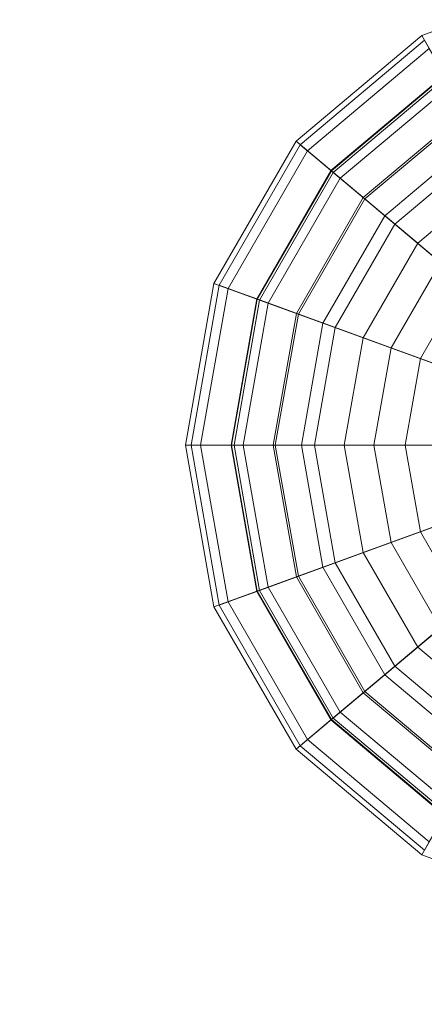
# Model space of a CAD drawing. Units: inches. Extents: x 375 to 1122, y 27 to 1069.
# Tile 97 of 155: x 717.434 to 718.593, y 863.668 to 866.486. Entities that reach past the tile are written whole.
import ezdxf

# ---------------------------------------------------------------- set-up
doc = ezdxf.new("R2010")
doc.units = ezdxf.units.IN
doc.layers.add('A-ANNO-DIMS', color=2, linetype='Continuous', lineweight=18)
doc.layers.add('Furniture', color=30, linetype='Continuous', lineweight=18)
doc.styles.get("Standard").update_dxf_attribs({"font": 'arial.ttf'})
doc.dimstyles.new('ISO-25', dxfattribs={"dimtxt": 12, "dimasz": 2.5, "dimexe": 1.5, "dimexo": 1.5, "dimtad": 1, "dimdec": 1, "dimlunit": 3, "dimtxsty": 'Standard', "dimblk": 'ARCHTICK', "dimcen": 2.5, "dimadec": 0, "dimazin": 0, "dimtfac": 1, "dimtdec": 1, "dimtmove": 0, "dimatfit": 3, "dimfxl": 1.5, "dimfxlon": 1, "dimarcsym": 0})

# ---------------------------------------------------------------- blocks, each defined once
blk = doc.blocks.new('A$C403C54AD')
for points in [[(1.793211, 0.852004, -0.031825), (1.826559, 0.857884, -0.028747), (1.826559, 0.857884, -0.028747), (1.797233, 0.840953, -0.031825)], [(1.797233, 0.840953, -0.031825), (1.826559, 0.857884, -0.028747), (1.826559, 0.857884, -0.028747), (1.804793, 0.831944, -0.031825)], [(1.804793, 0.831944, -0.031825), (1.826559, 0.857884, -0.028747), (1.826559, 0.857884, -0.028747), (1.814977, 0.826064, -0.031825)], [(1.814977, 0.826064, -0.031825), (1.826559, 0.857884, -0.028747), (1.826559, 0.857884, -0.028747), (1.826559, 0.824022, -0.031825)], [(1.855884, 0.840953, -0.031825), (1.826559, 0.857884, -0.028747), (1.826559, 0.857884, -0.028747), (1.859907, 0.852004, -0.031825)], [(1.848325, 0.831944, -0.031825), (1.826559, 0.857884, -0.028747), (1.826559, 0.857884, -0.028747), (1.855884, 0.840953, -0.031825)], [(1.83814, 0.826064, -0.031825), (1.826559, 0.857884, -0.028747), (1.826559, 0.857884, -0.028747), (1.848325, 0.831944, -0.031825)], [(1.826559, 0.824022, -0.031825), (1.826559, 0.857884, -0.028747), (1.826559, 0.857884, -0.028747), (1.83814, 0.826064, -0.031825)], [(1.796427, 0.852571, -0.028594), (1.793211, 0.852004, -0.031825), (1.797233, 0.840953, -0.031825), (1.800062, 0.842586, -0.028594)], [(1.853056, 0.842586, -0.028594), (1.855884, 0.840953, -0.031825), (1.859907, 0.852004, -0.031825), (1.85669, 0.852571, -0.028594)], [(1.814249, 0.850777, -0.02532), (1.800062, 0.842586, -0.028594), (1.806892, 0.834446, -0.028594), (1.817422, 0.846995, -0.02532)], [(1.820835, 0.851063, 0.057003), (1.814907, 0.843998, 0.063639), (1.820359, 0.84085, 0.063639), (1.823514, 0.849517, 0.057003)], [(1.829604, 0.849517, 0.057003), (1.832759, 0.84085, 0.063639), (1.838211, 0.843998, 0.063639), (1.832282, 0.851063, 0.057003)], [(1.835696, 0.846995, -0.02532), (1.846226, 0.834446, -0.028594), (1.853056, 0.842586, -0.028594), (1.838869, 0.850777, -0.02532)], [(1.813473, 0.842289, 0.061451), (1.820055, 0.850133, 0.054084), (1.823098, 0.848375, 0.054084), (1.819596, 0.838754, 0.061451)], [(1.833522, 0.838754, 0.061451), (1.83002, 0.848375, 0.054084), (1.833063, 0.850133, 0.054084), (1.839644, 0.842289, 0.061451)], [(1.823514, 0.849517, 0.057003), (1.820359, 0.84085, 0.063639), (1.826559, 0.839757, 0.063639), (1.826559, 0.84898, 0.057003)], [(1.826559, 0.84898, 0.057003), (1.826559, 0.839757, 0.063639), (1.832759, 0.84085, 0.063639), (1.829604, 0.849517, 0.057003)], [(1.81086, 0.84882, 0.063639), (1.805243, 0.845577, 0.073031), (1.810738, 0.839029, 0.073031), (1.814907, 0.843998, 0.063639)], [(1.838211, 0.843998, 0.063639), (1.84238, 0.839029, 0.073031), (1.847874, 0.845577, 0.073031), (1.842258, 0.84882, 0.063639)], [(1.819596, 0.838754, 0.061451), (1.823098, 0.848375, 0.054084), (1.826559, 0.847765, 0.054084), (1.826559, 0.837526, 0.061451)], [(1.826559, 0.837526, 0.061451), (1.826559, 0.847765, 0.054084), (1.83002, 0.848375, 0.054084), (1.833522, 0.838754, 0.061451)], [(1.802809, 0.844172, 0.071684), (1.808929, 0.847705, 0.061451), (1.813473, 0.842289, 0.061451), (1.808931, 0.836876, 0.071684)], [(1.844187, 0.836876, 0.071684), (1.839644, 0.842289, 0.061451), (1.844189, 0.847705, 0.061451), (1.850309, 0.844172, 0.071684)], [(1.802683, 0.844099, 0.130354), (1.80709, 0.846643, 0.140564), (1.812108, 0.840662, 0.140564), (1.808838, 0.836765, 0.130354)], [(1.80709, 0.846643, 0.140564), (1.804424, 0.845104, 0.140564), (1.81013, 0.838304, 0.140564), (1.812108, 0.840662, 0.140564)], [(1.817422, 0.846995, -0.02532), (1.806892, 0.834446, -0.028594), (1.816094, 0.829133, -0.028594), (1.821697, 0.844527, -0.02532)], [(1.83142, 0.844527, -0.02532), (1.837023, 0.829133, -0.028594), (1.846226, 0.834446, -0.028594), (1.835696, 0.846995, -0.02532)], [(1.84101, 0.840662, 0.140564), (1.842988, 0.838304, 0.140564), (1.848694, 0.845104, 0.140564), (1.846028, 0.846643, 0.140564)], [(1.84428, 0.836765, 0.130354), (1.84101, 0.840662, 0.140564), (1.846028, 0.846643, 0.140564), (1.850434, 0.844099, 0.130354)], [(1.804424, 0.845104, 0.140564), (1.800097, 0.842606, 0.131159), (1.806918, 0.834477, 0.131159), (1.81013, 0.838304, 0.140564)], [(1.805243, 0.845577, 0.073031), (1.80082, 0.843024, 0.090178), (1.807455, 0.835117, 0.090178), (1.810738, 0.839029, 0.073031)], [(1.84238, 0.839029, 0.073031), (1.845663, 0.835117, 0.090178), (1.852298, 0.843024, 0.090178), (1.847874, 0.845577, 0.073031)], [(1.842988, 0.838304, 0.140564), (1.8462, 0.834477, 0.131159), (1.853021, 0.842606, 0.131159), (1.848694, 0.845104, 0.140564)], [(1.821697, 0.844527, -0.02532), (1.816094, 0.829133, -0.028594), (1.826559, 0.827288, -0.028594), (1.826559, 0.84367, -0.02532)], [(1.826559, 0.84367, -0.02532), (1.826559, 0.827288, -0.028594), (1.837023, 0.829133, -0.028594), (1.83142, 0.844527, -0.02532)], [(1.798163, 0.84149, 0.089693), (1.802809, 0.844172, 0.071684), (1.808931, 0.836876, 0.071684), (1.805483, 0.832767, 0.089693)], [(1.80025, 0.842695, 0.117718), (1.802683, 0.844099, 0.130354), (1.808838, 0.836765, 0.130354), (1.807032, 0.834612, 0.117718)], [(1.814907, 0.843998, 0.063639), (1.810738, 0.839029, 0.073031), (1.818141, 0.834755, 0.073031), (1.820359, 0.84085, 0.063639)], [(1.832759, 0.84085, 0.063639), (1.834977, 0.834755, 0.073031), (1.84238, 0.839029, 0.073031), (1.838211, 0.843998, 0.063639)], [(1.847635, 0.832767, 0.089693), (1.844187, 0.836876, 0.071684), (1.850309, 0.844172, 0.071684), (1.854954, 0.84149, 0.089693)], [(1.846086, 0.834612, 0.117718), (1.84428, 0.836765, 0.130354), (1.850434, 0.844099, 0.130354), (1.852868, 0.842695, 0.117718)], [(1.80082, 0.843024, 0.090178), (1.80025, 0.842695, 0.117718), (1.807032, 0.834612, 0.117718), (1.807455, 0.835117, 0.090178)], [(1.845663, 0.835117, 0.090178), (1.846086, 0.834612, 0.117718), (1.852868, 0.842695, 0.117718), (1.852298, 0.843024, 0.090178)], [(1.800062, 0.842586, -0.028594), (1.797233, 0.840953, -0.031825), (1.804793, 0.831944, -0.031825), (1.806892, 0.834446, -0.028594)], [(1.800097, 0.842606, 0.131159), (1.797579, 0.841152, 0.117935), (1.805049, 0.83225, 0.117935), (1.806918, 0.834477, 0.131159)], [(1.808931, 0.836876, 0.071684), (1.813473, 0.842289, 0.061451), (1.819596, 0.838754, 0.061451), (1.817179, 0.832114, 0.071684)], [(1.835938, 0.832114, 0.071684), (1.833522, 0.838754, 0.061451), (1.839644, 0.842289, 0.061451), (1.844187, 0.836876, 0.071684)], [(1.8462, 0.834477, 0.131159), (1.848069, 0.83225, 0.117935), (1.855539, 0.841152, 0.117935), (1.853021, 0.842606, 0.131159)], [(1.846226, 0.834446, -0.028594), (1.848325, 0.831944, -0.031825), (1.855884, 0.840953, -0.031825), (1.853056, 0.842586, -0.028594)], [(1.797579, 0.841152, 0.117935), (1.798163, 0.84149, 0.089693), (1.805483, 0.832767, 0.089693), (1.805049, 0.83225, 0.117935)], [(1.820359, 0.84085, 0.063639), (1.818141, 0.834755, 0.073031), (1.826559, 0.833271, 0.073031), (1.826559, 0.839757, 0.063639)], [(1.826559, 0.839757, 0.063639), (1.826559, 0.833271, 0.073031), (1.834977, 0.834755, 0.073031), (1.832759, 0.84085, 0.063639)], [(1.848069, 0.83225, 0.117935), (1.847635, 0.832767, 0.089693), (1.854954, 0.84149, 0.089693), (1.855539, 0.841152, 0.117935)], [(1.808838, 0.836765, 0.130354), (1.812108, 0.840662, 0.140564), (1.81887, 0.836759, 0.140564), (1.81713, 0.831977, 0.130354)], [(1.812108, 0.840662, 0.140564), (1.81013, 0.838304, 0.140564), (1.817817, 0.833866, 0.140564), (1.81887, 0.836759, 0.140564)], [(1.834248, 0.836759, 0.140564), (1.835301, 0.833866, 0.140564), (1.842988, 0.838304, 0.140564), (1.84101, 0.840662, 0.140564)], [(1.835988, 0.831977, 0.130354), (1.834248, 0.836759, 0.140564), (1.84101, 0.840662, 0.140564), (1.84428, 0.836765, 0.130354)], [(1.810738, 0.839029, 0.073031), (1.807455, 0.835117, 0.090178), (1.816394, 0.829956, 0.090178), (1.818141, 0.834755, 0.073031)], [(1.817179, 0.832114, 0.071684), (1.819596, 0.838754, 0.061451), (1.826559, 0.837526, 0.061451), (1.826559, 0.83046, 0.071684)], [(1.826559, 0.83046, 0.071684), (1.826559, 0.837526, 0.061451), (1.833522, 0.838754, 0.061451), (1.835938, 0.832114, 0.071684)], [(1.834977, 0.834755, 0.073031), (1.836724, 0.829956, 0.090178), (1.845663, 0.835117, 0.090178), (1.84238, 0.839029, 0.073031)], [(1.81013, 0.838304, 0.140564), (1.806918, 0.834477, 0.131159), (1.816108, 0.829171, 0.131159), (1.817817, 0.833866, 0.140564)], [(1.835301, 0.833866, 0.140564), (1.83701, 0.829171, 0.131159), (1.8462, 0.834477, 0.131159), (1.842988, 0.838304, 0.140564)], [(1.805483, 0.832767, 0.089693), (1.808931, 0.836876, 0.071684), (1.817179, 0.832114, 0.071684), (1.815345, 0.827073, 0.089693)], [(1.807032, 0.834612, 0.117718), (1.808838, 0.836765, 0.130354), (1.81713, 0.831977, 0.130354), (1.816169, 0.829337, 0.117718)], [(1.81713, 0.831977, 0.130354), (1.81887, 0.836759, 0.140564), (1.826559, 0.835403, 0.140564), (1.826559, 0.830315, 0.130354)], [(1.81887, 0.836759, 0.140564), (1.817817, 0.833866, 0.140564), (1.826559, 0.832324, 0.140564), (1.826559, 0.835403, 0.140564)], [(1.826559, 0.835403, 0.140564), (1.826559, 0.832324, 0.140564), (1.835301, 0.833866, 0.140564), (1.834248, 0.836759, 0.140564)], [(1.826559, 0.830315, 0.130354), (1.826559, 0.835403, 0.140564), (1.834248, 0.836759, 0.140564), (1.835988, 0.831977, 0.130354)], [(1.837773, 0.827073, 0.089693), (1.835938, 0.832114, 0.071684), (1.844187, 0.836876, 0.071684), (1.847635, 0.832767, 0.089693)], [(1.836949, 0.829337, 0.117718), (1.835988, 0.831977, 0.130354), (1.84428, 0.836765, 0.130354), (1.846086, 0.834612, 0.117718)], [(1.806892, 0.834446, -0.028594), (1.804793, 0.831944, -0.031825), (1.814977, 0.826064, -0.031825), (1.816094, 0.829133, -0.028594)], [(1.806918, 0.834477, 0.131159), (1.805049, 0.83225, 0.117935), (1.815114, 0.826439, 0.117935), (1.816108, 0.829171, 0.131159)], [(1.807455, 0.835117, 0.090178), (1.807032, 0.834612, 0.117718), (1.816169, 0.829337, 0.117718), (1.816394, 0.829956, 0.090178)], [(1.818141, 0.834755, 0.073031), (1.816394, 0.829956, 0.090178), (1.826559, 0.828163, 0.090178), (1.826559, 0.833271, 0.073031)], [(1.826559, 0.833271, 0.073031), (1.826559, 0.828163, 0.090178), (1.836724, 0.829956, 0.090178), (1.834977, 0.834755, 0.073031)], [(1.836724, 0.829956, 0.090178), (1.836949, 0.829337, 0.117718), (1.846086, 0.834612, 0.117718), (1.845663, 0.835117, 0.090178)], [(1.83701, 0.829171, 0.131159), (1.838004, 0.826439, 0.117935), (1.848069, 0.83225, 0.117935), (1.8462, 0.834477, 0.131159)], [(1.837023, 0.829133, -0.028594), (1.83814, 0.826064, -0.031825), (1.848325, 0.831944, -0.031825), (1.846226, 0.834446, -0.028594)], [(1.817817, 0.833866, 0.140564), (1.816108, 0.829171, 0.131159), (1.826559, 0.827328, 0.131159), (1.826559, 0.832324, 0.140564)], [(1.826559, 0.832324, 0.140564), (1.826559, 0.827328, 0.131159), (1.83701, 0.829171, 0.131159), (1.835301, 0.833866, 0.140564)], [(1.805049, 0.83225, 0.117935), (1.805483, 0.832767, 0.089693), (1.815345, 0.827073, 0.089693), (1.815114, 0.826439, 0.117935)], [(1.838004, 0.826439, 0.117935), (1.837773, 0.827073, 0.089693), (1.847635, 0.832767, 0.089693), (1.848069, 0.83225, 0.117935)], [(1.815345, 0.827073, 0.089693), (1.817179, 0.832114, 0.071684), (1.826559, 0.83046, 0.071684), (1.826559, 0.825096, 0.089693)], [(1.816169, 0.829337, 0.117718), (1.81713, 0.831977, 0.130354), (1.826559, 0.830315, 0.130354), (1.826559, 0.827505, 0.117718)], [(1.826559, 0.825096, 0.089693), (1.826559, 0.83046, 0.071684), (1.835938, 0.832114, 0.071684), (1.837773, 0.827073, 0.089693)], [(1.826559, 0.827505, 0.117718), (1.826559, 0.830315, 0.130354), (1.835988, 0.831977, 0.130354), (1.836949, 0.829337, 0.117718)], [(1.816394, 0.829956, 0.090178), (1.816169, 0.829337, 0.117718), (1.826559, 0.827505, 0.117718), (1.826559, 0.828163, 0.090178)], [(1.826559, 0.828163, 0.090178), (1.826559, 0.827505, 0.117718), (1.836949, 0.829337, 0.117718), (1.836724, 0.829956, 0.090178)], [(1.816094, 0.829133, -0.028594), (1.814977, 0.826064, -0.031825), (1.826559, 0.824022, -0.031825), (1.826559, 0.827288, -0.028594)], [(1.816108, 0.829171, 0.131159), (1.815114, 0.826439, 0.117935), (1.826559, 0.824421, 0.117935), (1.826559, 0.827328, 0.131159)], [(1.826559, 0.827328, 0.131159), (1.826559, 0.824421, 0.117935), (1.838004, 0.826439, 0.117935), (1.83701, 0.829171, 0.131159)], [(1.826559, 0.827288, -0.028594), (1.826559, 0.824022, -0.031825), (1.83814, 0.826064, -0.031825), (1.837023, 0.829133, -0.028594)], [(1.815114, 0.826439, 0.117935), (1.815345, 0.827073, 0.089693), (1.826559, 0.825096, 0.089693), (1.826559, 0.824421, 0.117935)], [(1.826559, 0.824421, 0.117935), (1.826559, 0.825096, 0.089693), (1.837773, 0.827073, 0.089693), (1.838004, 0.826439, 0.117935)]]:
    blk.add_3dface(points)
blk = doc.blocks.new('_ArchTick')
at = {"color": 0, "linetype": 'ByBlock', "const_width": 0.15}
blk.add_lwpolyline([(-0.5, -0.5), (0.5, 0.5)], dxfattribs=at)
blk = doc.blocks.new('*D85')
at = {"layer": 'A-ANNO-DIMS', "color": 0, "lineweight": -2, "transparency": 16777216}
for p, q in [((401.5073, 868.5277), (398.5073, 868.5277)), ((400.0073, 814.5277), (400.0073, 868.5277)), ((401.5073, 814.5277), (398.5073, 814.5277))]:
    blk.add_line(p, q, dxfattribs=at)
at = {"layer": 'Defpoints', "color": 0, "transparency": 16777216}
for p in [(400.0073, 868.5277), (845.0073, 868.5277), (845.0073, 814.5277)]:
    blk.add_point(p, dxfattribs=at)
at = {"layer": 'A-ANNO-DIMS', "color": 0, "lineweight": -2, "transparency": 16777216, "xscale": 2.5, "yscale": 2.5, "zscale": 2.5}
for p, rotation in [((400.0073, 868.5277), 90), ((400.0073, 814.5277), 270)]:
    blk.add_blockref('_ArchTick', p, dxfattribs=dict(at, rotation=rotation))
at = {"layer": 'A-ANNO-DIMS', "color": 0, "transparency": 16777216, "insert": (393.2555, 841.5277), "char_height": 12, "attachment_point": 5, "rotation": 90}
blk.add_mtext('4\'-6"', dxfattribs=at)

msp = doc.modelspace()

# ---------------------------------------------------------------- block references
at = {"layer": 'Furniture', "xscale": 39.9918517141215, "yscale": 39.9918517141215, "zscale": 39.9918517141215, "rotation": 270}
msp.add_blockref('A$C403C54AD', (684.9549, 938.3156, 0.024), dxfattribs=at)

# ---------------------------------------------------------------- dimensions: what is measured, and where the dimension line sits
at = {"layer": 'A-ANNO-DIMS'}
dim = msp.add_linear_dim(base=(400.0073, 868.5277), p1=(845.0073, 814.5277), p2=(845.0073, 868.5277), angle=90, dimstyle='ISO-25', override={"dimdec": 1, "dimlfac": 1, "dimrnd": 0, "dimzin": 1, "dimdsep": 46, "dimlunit": 4, "dimfrac": 2}, dxfattribs=at)
dim.commit()
dim.dimension.update_dxf_attribs({"geometry": '*D85', "text_midpoint": (393.2555, 841.5277)})

doc.saveas('drawing.dxf')
